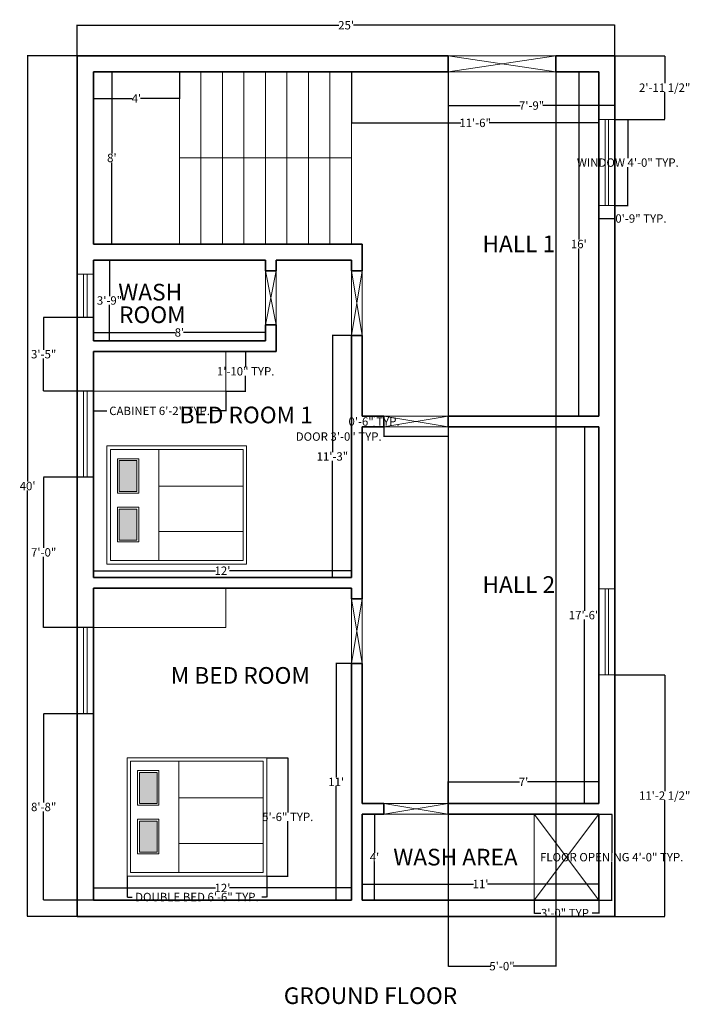
# Model space of a CAD drawing. Units: inches. Extents: x 292 to 2219, y -44 to 516.
# Tile 2 of 4: x 526 to 900, y -44 to 505. Entities that reach past the tile are written whole.
import ezdxf

# ---------------------------------------------------------------- set-up
doc = ezdxf.new("R2010")
doc.units = ezdxf.units.IN
doc.header["$MEASUREMENT"] = 0
for name, color, linetype, lineweight in [('A-ANNO-DIMS', 2, 'Continuous', 13), ('A-ANNO-TEXT', 7, 'Continuous', 25), ('A-AREA-IDEN', 7, 'Continuous', 18), ('A-DOOR', 34, 'Continuous', 20), ('A-FLOR-CASE', 9, 'Continuous', 18), ('A-FLOR-OPEN', 7, 'Continuous', 18), ('A-FLOR-STRS', 7, 'Continuous', 18), ('A-FURN', 8, 'Continuous', 18), ('A-GLAZ', 34, 'Continuous', 18), ('A-WALL', 7, 'Continuous', 35)]:
    doc.layers.add(name, color=color, linetype=linetype, lineweight=lineweight)
doc.styles.get("Standard").update_dxf_attribs({"font": 'arial.ttf'})
doc.dimstyles.get("Standard").update_dxf_attribs({"dimtxt": 4.68, "dimasz": 0.18, "dimexe": 0.18, "dimexo": 0.0625, "dimgap": 0.09, "dimtad": 0, "dimtih": 1, "dimtoh": 1, "dimdec": 0, "dimzin": 0, "dimdsep": 46, "dimlunit": 3, "dimtxsty": 'Standard', "dimcen": 0.09, "dimadec": 0, "dimazin": 0, "dimtfac": 1, "dimtdec": 0, "dimtofl": 0, "dimtmove": 0, "dimatfit": 3, "dimfxl": 1, "dimtolj": 1, "dimtzin": 0, "dimarcsym": 0})

# ---------------------------------------------------------------- blocks, each defined once
blk = doc.blocks.new('*D1')
at = {"layer": 'A-ANNO-DIMS', "color": 0, "lineweight": -2, "transparency": 16777216}
for p, q in [((558.22, 484.82), (530.37, 484.82)), ((530.55, 484.64), (530.55, 247.3)), ((530.55, 5), (530.55, 242.34)), ((558.22, 4.82), (530.37, 4.82))]:
    blk.add_line(p, q, dxfattribs=at)
at = {"layer": 'A-ANNO-DIMS', "color": 0, "transparency": 16777216}
for points in [[(530.52, 484.64), (530.58, 484.64), (530.55, 484.82)], [(530.52, 5), (530.58, 5), (530.55, 4.82)]]:
    blk.add_solid(points, dxfattribs=at)
at = {"layer": 'Defpoints', "color": 0, "transparency": 16777216}
for p in [(530.55, 484.82), (558.28, 484.82), (558.28, 4.82)]:
    blk.add_point(p, dxfattribs=at)
at = {"layer": 'A-ANNO-DIMS', "color": 0, "transparency": 16777216, "insert": (530.55, 244.82), "char_height": 4.68, "attachment_point": 5}
blk.add_mtext("\\A1;40'", dxfattribs=at)
blk = doc.blocks.new('*D2')
at = {"layer": 'A-ANNO-DIMS', "color": 0, "lineweight": -2, "transparency": 16777216}
for p, q in [((558.28, 484.88), (558.28, 502.04)), ((558.46, 501.86), (704.18, 501.86)), ((858.1, 501.86), (712.38, 501.86)), ((858.28, 484.88), (858.28, 502.04))]:
    blk.add_line(p, q, dxfattribs=at)
at = {"layer": 'A-ANNO-DIMS', "color": 0, "transparency": 16777216}
for points in [[(558.46, 501.89), (558.46, 501.83), (558.28, 501.86)], [(858.1, 501.89), (858.1, 501.83), (858.28, 501.86)]]:
    blk.add_solid(points, dxfattribs=at)
at = {"layer": 'Defpoints', "color": 0, "transparency": 16777216}
for p in [(858.28, 501.86), (558.28, 484.82), (858.28, 484.82)]:
    blk.add_point(p, dxfattribs=at)
at = {"layer": 'A-ANNO-DIMS', "color": 0, "transparency": 16777216, "insert": (708.28, 501.86), "char_height": 4.68, "attachment_point": 5}
blk.add_mtext("\\A1;25'", dxfattribs=at)
blk = doc.blocks.new('*D3')
at = {"layer": 'A-ANNO-DIMS', "color": 0, "lineweight": -2, "transparency": 16777216}
for p, q in [((849.22, 475.82), (837.97, 475.82)), ((838.15, 475.64), (838.15, 382.3)), ((838.15, 284), (838.15, 377.34)), ((849.22, 283.82), (837.97, 283.82))]:
    blk.add_line(p, q, dxfattribs=at)
at = {"layer": 'A-ANNO-DIMS', "color": 0, "transparency": 16777216}
for points in [[(838.12, 475.64), (838.18, 475.64), (838.15, 475.82)], [(838.12, 284), (838.18, 284), (838.15, 283.82)]]:
    blk.add_solid(points, dxfattribs=at)
at = {"layer": 'Defpoints', "color": 0, "transparency": 16777216}
for p in [(849.28, 475.82), (838.15, 283.82), (849.28, 283.82)]:
    blk.add_point(p, dxfattribs=at)
at = {"layer": 'A-ANNO-DIMS', "color": 0, "transparency": 16777216, "insert": (838.15, 379.82), "char_height": 4.68, "attachment_point": 5}
blk.add_mtext("\\A1;16'", dxfattribs=at)
blk = doc.blocks.new('*D4')
at = {"layer": 'A-ANNO-DIMS', "color": 0, "lineweight": -2, "transparency": 16777216}
for p, q in [((711.28, 475.75), (711.28, 447.21)), ((849.28, 475.75), (849.28, 447.21)), ((711.46, 447.39), (772.37, 447.39)), ((849.1, 447.39), (788.19, 447.39))]:
    blk.add_line(p, q, dxfattribs=at)
at = {"layer": 'A-ANNO-DIMS', "color": 0, "transparency": 16777216}
for points in [[(711.46, 447.42), (711.46, 447.36), (711.28, 447.39)], [(849.1, 447.42), (849.1, 447.36), (849.28, 447.39)]]:
    blk.add_solid(points, dxfattribs=at)
at = {"layer": 'Defpoints', "color": 0, "transparency": 16777216}
for p in [(711.28, 475.82), (849.28, 475.82), (849.28, 447.39)]:
    blk.add_point(p, dxfattribs=at)
at = {"layer": 'A-ANNO-DIMS', "color": 0, "transparency": 16777216, "insert": (780.28, 447.39), "char_height": 4.68, "attachment_point": 5}
blk.add_mtext('\\A1;11\'-6"', dxfattribs=at)
blk = doc.blocks.new('*D5')
at = {"layer": 'A-ANNO-DIMS', "color": 0, "lineweight": -2, "transparency": 16777216}
for p, q in [((567.28, 475.75), (567.28, 460.8)), ((615.28, 475.75), (615.28, 460.8)), ((567.46, 460.98), (588.94, 460.98)), ((615.1, 460.98), (593.62, 460.98))]:
    blk.add_line(p, q, dxfattribs=at)
at = {"layer": 'A-ANNO-DIMS', "color": 0, "transparency": 16777216}
for points in [[(567.46, 461.01), (567.46, 460.95), (567.28, 460.98)], [(615.1, 461.01), (615.1, 460.95), (615.28, 460.98)]]:
    blk.add_solid(points, dxfattribs=at)
at = {"layer": 'Defpoints', "color": 0, "transparency": 16777216}
for p in [(567.28, 475.82), (615.28, 475.82), (615.28, 460.98)]:
    blk.add_point(p, dxfattribs=at)
at = {"layer": 'A-ANNO-DIMS', "color": 0, "transparency": 16777216, "insert": (591.28, 460.98), "char_height": 4.68, "attachment_point": 5}
blk.add_mtext("\\A1;4'", dxfattribs=at)
blk = doc.blocks.new('*D6')
at = {"layer": 'A-ANNO-DIMS', "color": 0, "lineweight": -2, "transparency": 16777216}
for p, q in [((567.34, 475.82), (577.74, 475.82)), ((577.56, 475.64), (577.56, 430.3)), ((577.56, 380), (577.56, 425.34)), ((567.34, 379.82), (577.74, 379.82))]:
    blk.add_line(p, q, dxfattribs=at)
at = {"layer": 'A-ANNO-DIMS', "color": 0, "transparency": 16777216}
for points in [[(577.53, 475.64), (577.59, 475.64), (577.56, 475.82)], [(577.53, 380), (577.59, 380), (577.56, 379.82)]]:
    blk.add_solid(points, dxfattribs=at)
at = {"layer": 'Defpoints', "color": 0, "transparency": 16777216}
for p in [(567.28, 475.82), (567.28, 379.82), (577.56, 379.82)]:
    blk.add_point(p, dxfattribs=at)
at = {"layer": 'A-ANNO-DIMS', "color": 0, "transparency": 16777216, "insert": (577.56, 427.82), "char_height": 4.68, "attachment_point": 5}
blk.add_mtext("\\A1;8'", dxfattribs=at)
blk = doc.blocks.new('*D7')
at = {"layer": 'A-ANNO-DIMS', "color": 0, "lineweight": -2, "transparency": 16777216}
for p, q in [((567.28, 325.88), (567.28, 330.66)), ((567.46, 330.48), (613.03, 330.48)), ((663.1, 330.48), (617.52, 330.48)), ((663.28, 325.88), (663.28, 330.66))]:
    blk.add_line(p, q, dxfattribs=at)
at = {"layer": 'A-ANNO-DIMS', "color": 0, "transparency": 16777216}
for points in [[(567.46, 330.51), (567.46, 330.45), (567.28, 330.48)], [(663.1, 330.51), (663.1, 330.45), (663.28, 330.48)]]:
    blk.add_solid(points, dxfattribs=at)
at = {"layer": 'Defpoints', "color": 0, "transparency": 16777216}
for p in [(663.28, 330.48), (567.28, 325.82), (663.28, 325.82)]:
    blk.add_point(p, dxfattribs=at)
at = {"layer": 'A-ANNO-DIMS', "color": 0, "transparency": 16777216, "insert": (615.28, 330.48), "char_height": 4.68, "attachment_point": 5}
blk.add_mtext("\\A1;8'", dxfattribs=at)
blk = doc.blocks.new('*D8')
at = {"layer": 'A-ANNO-DIMS', "color": 0, "lineweight": -2, "transparency": 16777216}
for p, q in [((567.34, 370.82), (576.43, 370.82)), ((576.25, 370.64), (576.25, 350.8)), ((576.25, 326), (576.25, 345.84)), ((567.34, 325.82), (576.43, 325.82))]:
    blk.add_line(p, q, dxfattribs=at)
at = {"layer": 'A-ANNO-DIMS', "color": 0, "transparency": 16777216}
for points in [[(576.22, 370.64), (576.28, 370.64), (576.25, 370.82)], [(576.22, 326), (576.28, 326), (576.25, 325.82)]]:
    blk.add_solid(points, dxfattribs=at)
at = {"layer": 'Defpoints', "color": 0, "transparency": 16777216}
for p in [(567.28, 370.82), (576.25, 370.82), (567.28, 325.82)]:
    blk.add_point(p, dxfattribs=at)
at = {"layer": 'A-ANNO-DIMS', "color": 0, "transparency": 16777216, "insert": (576.25, 348.32), "char_height": 4.68, "attachment_point": 5}
blk.add_mtext('\\A1;3\'-9"', dxfattribs=at)
blk = doc.blocks.new('*D9')
at = {"layer": 'A-ANNO-DIMS', "color": 0, "lineweight": -2, "transparency": 16777216}
for p, q in [((711.22, 328.82), (700.45, 328.82)), ((700.63, 328.64), (700.63, 263.8)), ((700.63, 194), (700.63, 258.84)), ((711.22, 193.82), (700.45, 193.82))]:
    blk.add_line(p, q, dxfattribs=at)
at = {"layer": 'A-ANNO-DIMS', "color": 0, "transparency": 16777216}
for points in [[(700.6, 328.64), (700.66, 328.64), (700.63, 328.82)], [(700.6, 194), (700.66, 194), (700.63, 193.82)]]:
    blk.add_solid(points, dxfattribs=at)
at = {"layer": 'Defpoints', "color": 0, "transparency": 16777216}
for p in [(700.63, 328.82), (711.28, 328.82), (711.28, 193.82)]:
    blk.add_point(p, dxfattribs=at)
at = {"layer": 'A-ANNO-DIMS', "color": 0, "transparency": 16777216, "insert": (700.63, 261.32), "char_height": 4.68, "attachment_point": 5}
blk.add_mtext('\\A1;11\'-3"', dxfattribs=at)
blk = doc.blocks.new('*D10')
at = {"layer": 'A-ANNO-DIMS', "color": 0, "lineweight": -2, "transparency": 16777216}
for p, q in [((567.28, 193.88), (567.28, 197.79)), ((711.28, 193.88), (711.28, 197.79)), ((567.46, 197.61), (635.44, 197.61)), ((711.1, 197.61), (643.12, 197.61))]:
    blk.add_line(p, q, dxfattribs=at)
at = {"layer": 'A-ANNO-DIMS', "color": 0, "transparency": 16777216}
for points in [[(567.46, 197.64), (567.46, 197.58), (567.28, 197.61)], [(711.1, 197.64), (711.1, 197.58), (711.28, 197.61)]]:
    blk.add_solid(points, dxfattribs=at)
at = {"layer": 'Defpoints', "color": 0, "transparency": 16777216}
for p in [(567.28, 193.82), (711.28, 197.61), (711.28, 193.82)]:
    blk.add_point(p, dxfattribs=at)
at = {"layer": 'A-ANNO-DIMS', "color": 0, "transparency": 16777216, "insert": (639.28, 197.61), "char_height": 4.68, "attachment_point": 5}
blk.add_mtext("\\A1;12'", dxfattribs=at)
blk = doc.blocks.new('*D11')
at = {"layer": 'A-ANNO-DIMS', "color": 0, "lineweight": -2, "transparency": 16777216}
for p, q in [((567.28, 13.88), (567.28, 20.83)), ((567.46, 20.65), (635.44, 20.65)), ((711.1, 20.65), (643.12, 20.65)), ((711.28, 13.88), (711.28, 20.83))]:
    blk.add_line(p, q, dxfattribs=at)
at = {"layer": 'A-ANNO-DIMS', "color": 0, "transparency": 16777216}
for points in [[(567.46, 20.68), (567.46, 20.62), (567.28, 20.65)], [(711.1, 20.68), (711.1, 20.62), (711.28, 20.65)]]:
    blk.add_solid(points, dxfattribs=at)
at = {"layer": 'Defpoints', "color": 0, "transparency": 16777216}
for p in [(711.28, 20.65), (567.28, 13.82), (711.28, 13.82)]:
    blk.add_point(p, dxfattribs=at)
at = {"layer": 'A-ANNO-DIMS', "color": 0, "transparency": 16777216, "insert": (639.28, 20.65), "char_height": 4.68, "attachment_point": 5}
blk.add_mtext("\\A1;12'", dxfattribs=at)
blk = doc.blocks.new('*D12')
at = {"layer": 'A-ANNO-DIMS', "color": 0, "lineweight": -2, "transparency": 16777216}
for p, q in [((711.22, 145.82), (702.56, 145.82)), ((702.74, 145.64), (702.74, 82.26)), ((702.74, 14), (702.74, 77.38)), ((711.22, 13.82), (702.56, 13.82))]:
    blk.add_line(p, q, dxfattribs=at)
at = {"layer": 'A-ANNO-DIMS', "color": 0, "transparency": 16777216}
for points in [[(702.71, 145.64), (702.77, 145.64), (702.74, 145.82)], [(702.71, 14), (702.77, 14), (702.74, 13.82)]]:
    blk.add_solid(points, dxfattribs=at)
at = {"layer": 'Defpoints', "color": 0, "transparency": 16777216}
for p in [(702.74, 145.82), (711.28, 145.82), (711.28, 13.82)]:
    blk.add_point(p, dxfattribs=at)
at = {"layer": 'A-ANNO-DIMS', "color": 0, "transparency": 16777216, "insert": (702.74, 79.82), "char_height": 4.68, "attachment_point": 5}
blk.add_mtext("\\A1;11'", dxfattribs=at)
blk = doc.blocks.new('*D13')
at = {"layer": 'A-ANNO-DIMS', "color": 0, "lineweight": -2, "transparency": 16777216}
for p, q in [((717.28, 13.88), (717.28, 23.02)), ((717.46, 22.84), (779.44, 22.84)), ((849.1, 22.84), (787.12, 22.84)), ((849.28, 13.88), (849.28, 23.02))]:
    blk.add_line(p, q, dxfattribs=at)
at = {"layer": 'A-ANNO-DIMS', "color": 0, "transparency": 16777216}
for points in [[(717.46, 22.87), (717.46, 22.81), (717.28, 22.84)], [(849.1, 22.87), (849.1, 22.81), (849.28, 22.84)]]:
    blk.add_solid(points, dxfattribs=at)
at = {"layer": 'Defpoints', "color": 0, "transparency": 16777216}
for p in [(849.28, 22.84), (717.28, 13.82), (849.28, 13.82)]:
    blk.add_point(p, dxfattribs=at)
at = {"layer": 'A-ANNO-DIMS', "color": 0, "transparency": 16777216, "insert": (783.28, 22.84), "char_height": 4.68, "attachment_point": 5}
blk.add_mtext("\\A1;11'", dxfattribs=at)
blk = doc.blocks.new('*D14')
at = {"layer": 'A-ANNO-DIMS', "color": 0, "lineweight": -2, "transparency": 16777216}
for p, q in [((717.34, 61.82), (724.29, 61.82)), ((724.11, 61.64), (724.11, 40.25)), ((724.11, 14), (724.11, 35.39)), ((717.34, 13.82), (724.29, 13.82))]:
    blk.add_line(p, q, dxfattribs=at)
at = {"layer": 'A-ANNO-DIMS', "color": 0, "transparency": 16777216}
for points in [[(724.08, 61.64), (724.14, 61.64), (724.11, 61.82)], [(724.08, 14), (724.14, 14), (724.11, 13.82)]]:
    blk.add_solid(points, dxfattribs=at)
at = {"layer": 'Defpoints', "color": 0, "transparency": 16777216}
for p in [(717.28, 61.82), (717.28, 13.82), (724.11, 13.82)]:
    blk.add_point(p, dxfattribs=at)
at = {"layer": 'A-ANNO-DIMS', "color": 0, "transparency": 16777216, "insert": (724.11, 37.82), "char_height": 4.68, "attachment_point": 5}
blk.add_mtext("\\A1;4'", dxfattribs=at)
blk = doc.blocks.new('*D15')
at = {"layer": 'A-ANNO-DIMS', "color": 0, "lineweight": -2, "transparency": 16777216}
for p, q in [((849.22, 277.82), (841.19, 277.82)), ((841.37, 277.64), (841.37, 175.3)), ((841.37, 68), (841.37, 170.34)), ((849.22, 67.82), (841.19, 67.82))]:
    blk.add_line(p, q, dxfattribs=at)
at = {"layer": 'A-ANNO-DIMS', "color": 0, "transparency": 16777216}
for points in [[(841.34, 277.64), (841.4, 277.64), (841.37, 277.82)], [(841.34, 68), (841.4, 68), (841.37, 67.82)]]:
    blk.add_solid(points, dxfattribs=at)
at = {"layer": 'Defpoints', "color": 0, "transparency": 16777216}
for p in [(849.28, 277.82), (841.37, 67.82), (849.28, 67.82)]:
    blk.add_point(p, dxfattribs=at)
at = {"layer": 'A-ANNO-DIMS', "color": 0, "transparency": 16777216, "insert": (841.37, 172.82), "char_height": 4.68, "attachment_point": 5}
blk.add_mtext('\\A1;17\'-6"', dxfattribs=at)
blk = doc.blocks.new('*D16')
at = {"layer": 'A-ANNO-DIMS', "color": 0, "lineweight": -2, "transparency": 16777216}
for p, q in [((765.28, 67.88), (765.28, 79.96)), ((765.46, 79.78), (805.05, 79.78)), ((849.1, 79.78), (809.5, 79.78)), ((849.28, 67.88), (849.28, 79.96))]:
    blk.add_line(p, q, dxfattribs=at)
at = {"layer": 'A-ANNO-DIMS', "color": 0, "transparency": 16777216}
for points in [[(765.46, 79.81), (765.46, 79.75), (765.28, 79.78)], [(849.1, 79.81), (849.1, 79.75), (849.28, 79.78)]]:
    blk.add_solid(points, dxfattribs=at)
at = {"layer": 'Defpoints', "color": 0, "transparency": 16777216}
for p in [(849.28, 79.78), (765.28, 67.82), (849.28, 67.82)]:
    blk.add_point(p, dxfattribs=at)
at = {"layer": 'A-ANNO-DIMS', "color": 0, "transparency": 16777216, "insert": (807.28, 79.78), "char_height": 4.68, "attachment_point": 5}
blk.add_mtext("\\A1;7'", dxfattribs=at)
blk = doc.blocks.new('BED-DOUBLE')
h = blk.add_hatch(color=256)
h.dxf.hatch_style = 1
h.paths.add_polyline_path([(6.9, 40.51), (16.75, 40.51), (16.75, 57.79), (6.9, 57.79)])
h.paths.add_polyline_path([(16.75, 30.67), (6.9, 30.67), (6.9, 13.4), (16.75, 13.4)])
for p, q in [((0, 0), (0, 66)), ((0, 66), (78, 66)), ((78, 66), (78, 0)), ((2, 64), (76, 64)), ((2, 2), (2, 64)), ((29, 2), (29, 64)), ((76, 64), (76, 2)), ((76, 43.53), (29, 43.53)), ((76, 18.22), (29, 18.22)), ((78, 0), (0, 0)), ((76, 2), (2, 2))]:
    blk.add_line(p, q)
for points in [[(5.9, 58.79), (17.75, 58.79), (17.75, 39.51), (5.9, 39.51)], [(6.9, 57.79), (16.75, 57.79), (16.75, 40.51), (6.9, 40.51)], [(5.9, 31.67), (17.75, 31.67), (17.75, 12.4), (5.9, 12.4)], [(6.9, 30.67), (16.75, 30.67), (16.75, 13.4), (6.9, 13.4)]]:
    blk.add_lwpolyline(points, close=True)
blk = doc.blocks.new('WIN-48')
for p, q in [((0, 48), (9, 48)), ((0, 0), (0, 48)), ((3.5, 48), (3.5, 0)), ((5.5, 48), (5.5, 0)), ((9, 48), (9, 0)), ((9, 0), (0, 0))]:
    blk.add_line(p, q)
blk = doc.blocks.new('DOOR-36')
for p, q in [((0, 36), (6, 36)), ((0, 0), (6, 36)), ((6, 0), (0, 36)), ((0, 36), (0, 0)), ((6, 36), (6, 0)), ((0, 0), (6, 0))]:
    blk.add_line(p, q)
blk = doc.blocks.new('WIN-24')
for p, q in [((0, 24), (9, 24)), ((0, 24), (0, 0)), ((3.5, 24), (3.5, 0)), ((5.5, 24), (5.5, 0)), ((9, 24), (9, 0)), ((0, 0), (9, 0))]:
    blk.add_line(p, q)
blk = doc.blocks.new('DOOR-30')
for p, q in [((0, 30), (6, 30)), ((0, 30), (6, 0)), ((6, 30), (0, 0)), ((0, 0), (0, 30)), ((6, 0), (6, 30)), ((0, 0), (6, 0))]:
    blk.add_line(p, q)
blk = doc.blocks.new('FLOOR-OPENING-36X48')
for p, q in [((0, 48), (0, 0)), ((0, 48), (36, 0)), ((36, 48), (0, 0))]:
    blk.add_line(p, q)
blk = doc.blocks.new('BEDROOM-CABINET')
blk.add_lwpolyline([(0, 21.98), (73.86, 21.98), (73.86, 0), (0, 0)], close=True)
blk = doc.blocks.new('*D44')
at = {"layer": 'A-ANNO-DIMS', "color": 0, "lineweight": -2, "transparency": 16777216}
for p, q in [((858.34, 449.23), (865.66, 449.23)), ((865.48, 449.05), (865.48, 427.74)), ((865.48, 401.41), (865.48, 422.72)), ((858.34, 401.23), (865.66, 401.23))]:
    blk.add_line(p, q, dxfattribs=at)
at = {"layer": 'A-ANNO-DIMS', "color": 0, "transparency": 16777216}
for points in [[(865.45, 449.05), (865.51, 449.05), (865.48, 449.23)], [(865.45, 401.41), (865.51, 401.41), (865.48, 401.23)]]:
    blk.add_solid(points, dxfattribs=at)
at = {"layer": 'Defpoints', "color": 0, "transparency": 16777216}
for p in [(858.28, 449.23), (865.48, 449.23), (858.28, 401.23)]:
    blk.add_point(p, dxfattribs=at)
at = {"layer": 'A-ANNO-DIMS', "color": 0, "transparency": 16777216, "insert": (865.48, 425.23), "char_height": 4.68, "attachment_point": 5}
blk.add_mtext('\\A1;WINDOW 4\'-0" TYP.', dxfattribs=at)
blk = doc.blocks.new('*D45')
at = {"layer": 'A-ANNO-DIMS', "color": 0, "lineweight": -2, "transparency": 16777216}
for p, q in [((849.28, 401.17), (849.28, 393.85)), ((858.28, 401.17), (858.28, 393.85)), ((849.46, 394.03), (858.1, 394.03)), ((858.28, 394.03), (858.46, 394.03))]:
    blk.add_line(p, q, dxfattribs=at)
at = {"layer": 'A-ANNO-DIMS', "color": 0, "transparency": 16777216}
for points in [[(849.46, 394.06), (849.46, 394), (849.28, 394.03)], [(858.1, 394.06), (858.1, 394), (858.28, 394.03)]]:
    blk.add_solid(points, dxfattribs=at)
at = {"layer": 'Defpoints', "color": 0, "transparency": 16777216}
for p in [(849.28, 401.23), (858.28, 401.23), (858.28, 394.03)]:
    blk.add_point(p, dxfattribs=at)
at = {"layer": 'A-ANNO-DIMS', "color": 0, "transparency": 16777216, "insert": (872.81, 394.03), "char_height": 4.68, "attachment_point": 5}
blk.add_mtext('\\A1;0\'-9" TYP.', dxfattribs=at)
blk = doc.blocks.new('*D48')
at = {"layer": 'A-ANNO-DIMS', "color": 0, "lineweight": -2, "transparency": 16777216}
for p, q in [((729.28, 277.75), (729.28, 272.24)), ((765.28, 277.75), (765.28, 272.24)), ((729.28, 272.42), (729.1, 272.42)), ((765.1, 272.42), (729.46, 272.42))]:
    blk.add_line(p, q, dxfattribs=at)
at = {"layer": 'A-ANNO-DIMS', "color": 0, "transparency": 16777216}
for points in [[(729.46, 272.45), (729.46, 272.39), (729.28, 272.42)], [(765.1, 272.45), (765.1, 272.39), (765.28, 272.42)]]:
    blk.add_solid(points, dxfattribs=at)
at = {"layer": 'Defpoints', "color": 0, "transparency": 16777216}
for p in [(729.28, 277.82), (765.28, 277.82), (729.28, 272.42)]:
    blk.add_point(p, dxfattribs=at)
at = {"layer": 'A-ANNO-DIMS', "color": 0, "transparency": 16777216, "insert": (704.15, 272.42), "char_height": 4.68, "attachment_point": 5}
blk.add_mtext('\\A1;DOOR 3\'-0" TYP.', dxfattribs=at)
blk = doc.blocks.new('*D49')
at = {"layer": 'A-ANNO-DIMS', "color": 0, "lineweight": -2, "transparency": 16777216}
for p, q in [((729.22, 283.82), (723.7, 283.82)), ((723.88, 283.64), (723.88, 283.3)), ((729.22, 277.82), (723.7, 277.82)), ((723.88, 278), (723.88, 278.34))]:
    blk.add_line(p, q, dxfattribs=at)
at = {"layer": 'A-ANNO-DIMS', "color": 0, "transparency": 16777216}
for points in [[(723.85, 283.64), (723.91, 283.64), (723.88, 283.82)], [(723.85, 278), (723.91, 278), (723.88, 277.82)]]:
    blk.add_solid(points, dxfattribs=at)
at = {"layer": 'Defpoints', "color": 0, "transparency": 16777216}
for p in [(723.88, 283.82), (729.28, 283.82), (729.28, 277.82)]:
    blk.add_point(p, dxfattribs=at)
at = {"layer": 'A-ANNO-DIMS', "color": 0, "transparency": 16777216, "insert": (723.88, 280.82), "char_height": 4.68, "attachment_point": 5}
blk.add_mtext('\\A1;0\'-6" TYP.', dxfattribs=at)
blk = doc.blocks.new('*D52')
at = {"layer": 'A-ANNO-DIMS', "color": 0, "lineweight": -2, "transparency": 16777216}
for p, q in [((586.02, 27.24), (586.02, 15.42)), ((664.02, 27.24), (664.02, 15.42)), ((586.2, 15.6), (588.8, 15.6)), ((663.84, 15.6), (661.24, 15.6))]:
    blk.add_line(p, q, dxfattribs=at)
at = {"layer": 'A-ANNO-DIMS', "color": 0, "transparency": 16777216}
for points in [[(586.2, 15.63), (586.2, 15.57), (586.02, 15.6)], [(663.84, 15.63), (663.84, 15.57), (664.02, 15.6)]]:
    blk.add_solid(points, dxfattribs=at)
at = {"layer": 'Defpoints', "color": 0, "transparency": 16777216}
for p in [(586.02, 27.3), (664.02, 27.3), (664.02, 15.6)]:
    blk.add_point(p, dxfattribs=at)
at = {"layer": 'A-ANNO-DIMS', "color": 0, "transparency": 16777216, "insert": (625.02, 15.6), "char_height": 4.68, "attachment_point": 5}
blk.add_mtext('\\A1;DOUBLE BED 6\'-6" TYP.', dxfattribs=at)
blk = doc.blocks.new('*D53')
at = {"layer": 'A-ANNO-DIMS', "color": 0, "lineweight": -2, "transparency": 16777216}
for p, q in [((664.08, 93.3), (675.9, 93.3)), ((675.72, 93.12), (675.72, 62.78)), ((675.72, 27.48), (675.72, 57.82)), ((664.08, 27.3), (675.9, 27.3))]:
    blk.add_line(p, q, dxfattribs=at)
at = {"layer": 'A-ANNO-DIMS', "color": 0, "transparency": 16777216}
for points in [[(675.69, 93.12), (675.75, 93.12), (675.72, 93.3)], [(675.69, 27.48), (675.75, 27.48), (675.72, 27.3)]]:
    blk.add_solid(points, dxfattribs=at)
at = {"layer": 'Defpoints', "color": 0, "transparency": 16777216}
for p in [(664.02, 93.3), (675.72, 93.3), (664.02, 27.3)]:
    blk.add_point(p, dxfattribs=at)
at = {"layer": 'A-ANNO-DIMS', "color": 0, "transparency": 16777216, "insert": (675.72, 60.3), "char_height": 4.68, "attachment_point": 5}
blk.add_mtext('\\A1;5\'-6" TYP.', dxfattribs=at)
blk = doc.blocks.new('*D54')
at = {"layer": 'A-ANNO-DIMS', "color": 0, "lineweight": -2, "transparency": 16777216}
for p, q in [((567.28, 297.77), (567.28, 286.57)), ((641.14, 297.77), (641.14, 286.57)), ((567.46, 286.75), (574.81, 286.75)), ((640.96, 286.75), (633.61, 286.75))]:
    blk.add_line(p, q, dxfattribs=at)
at = {"layer": 'A-ANNO-DIMS', "color": 0, "transparency": 16777216}
for points in [[(567.46, 286.78), (567.46, 286.72), (567.28, 286.75)], [(640.96, 286.78), (640.96, 286.72), (641.14, 286.75)]]:
    blk.add_solid(points, dxfattribs=at)
at = {"layer": 'Defpoints', "color": 0, "transparency": 16777216}
for p in [(567.28, 297.83), (641.14, 297.83), (641.14, 286.75)]:
    blk.add_point(p, dxfattribs=at)
at = {"layer": 'A-ANNO-DIMS', "color": 0, "transparency": 16777216, "insert": (604.21, 286.75), "char_height": 4.68, "attachment_point": 5}
blk.add_mtext('\\A1;CABINET 6\'-2" TYP.', dxfattribs=at)
blk = doc.blocks.new('*D55')
at = {"layer": 'A-ANNO-DIMS', "color": 0, "lineweight": -2, "transparency": 16777216}
for p, q in [((641.2, 319.82), (652.4, 319.82)), ((652.22, 319.64), (652.22, 311.3)), ((652.22, 298.01), (652.22, 306.34)), ((641.2, 297.83), (652.4, 297.83))]:
    blk.add_line(p, q, dxfattribs=at)
at = {"layer": 'A-ANNO-DIMS', "color": 0, "transparency": 16777216}
for points in [[(652.19, 319.64), (652.25, 319.64), (652.22, 319.82)], [(652.19, 298.01), (652.25, 298.01), (652.22, 297.83)]]:
    blk.add_solid(points, dxfattribs=at)
at = {"layer": 'Defpoints', "color": 0, "transparency": 16777216}
for p in [(641.14, 319.82), (652.22, 319.82), (641.14, 297.83)]:
    blk.add_point(p, dxfattribs=at)
at = {"layer": 'A-ANNO-DIMS', "color": 0, "transparency": 16777216, "insert": (652.22, 308.82), "char_height": 4.68, "attachment_point": 5}
blk.add_mtext('\\A1;1\'-10" TYP.', dxfattribs=at)
blk = doc.blocks.new('*D56')
at = {"layer": 'A-ANNO-DIMS', "color": 0, "lineweight": -2, "transparency": 16777216}
for p, q in [((849.34, 61.82), (856.66, 61.82)), ((856.48, 61.64), (856.48, 40.33)), ((856.48, 14), (856.48, 35.3)), ((849.34, 13.82), (856.66, 13.82))]:
    blk.add_line(p, q, dxfattribs=at)
at = {"layer": 'A-ANNO-DIMS', "color": 0, "transparency": 16777216}
for points in [[(856.45, 61.64), (856.51, 61.64), (856.48, 61.82)], [(856.45, 14), (856.51, 14), (856.48, 13.82)]]:
    blk.add_solid(points, dxfattribs=at)
at = {"layer": 'Defpoints', "color": 0, "transparency": 16777216}
for p in [(849.28, 61.82), (856.48, 61.82), (849.28, 13.82)]:
    blk.add_point(p, dxfattribs=at)
at = {"layer": 'A-ANNO-DIMS', "color": 0, "transparency": 16777216, "insert": (856.48, 37.82), "char_height": 4.68, "attachment_point": 5}
blk.add_mtext('\\A1;FLOOR OPENING 4\'-0" TYP.', dxfattribs=at)
blk = doc.blocks.new('*D57')
at = {"layer": 'A-ANNO-DIMS', "color": 0, "lineweight": -2, "transparency": 16777216}
for p, q in [((813.28, 13.75), (813.28, 6.44)), ((849.28, 13.75), (849.28, 6.44)), ((813.46, 6.62), (816.93, 6.62)), ((849.1, 6.62), (845.63, 6.62))]:
    blk.add_line(p, q, dxfattribs=at)
at = {"layer": 'A-ANNO-DIMS', "color": 0, "transparency": 16777216}
for points in [[(813.46, 6.65), (813.46, 6.59), (813.28, 6.62)], [(849.1, 6.65), (849.1, 6.59), (849.28, 6.62)]]:
    blk.add_solid(points, dxfattribs=at)
at = {"layer": 'Defpoints', "color": 0, "transparency": 16777216}
for p in [(813.28, 13.82), (849.28, 13.82), (849.28, 6.62)]:
    blk.add_point(p, dxfattribs=at)
at = {"layer": 'A-ANNO-DIMS', "color": 0, "transparency": 16777216, "insert": (831.28, 6.62), "char_height": 4.68, "attachment_point": 5}
blk.add_mtext('\\A1;3\'-0" TYP.', dxfattribs=at)
blk = doc.blocks.new('*D58')
at = {"layer": 'A-ANNO-DIMS', "color": 0, "lineweight": -2, "transparency": 16777216}
for p, q in [((765.28, 475.75), (765.28, -23.14)), ((825.28, 475.75), (825.28, -23.14)), ((765.46, -22.96), (788.97, -22.96)), ((825.1, -22.96), (801.59, -22.96))]:
    blk.add_line(p, q, dxfattribs=at)
at = {"layer": 'A-ANNO-DIMS', "color": 0, "transparency": 16777216}
for points in [[(765.46, -22.93), (765.46, -22.99), (765.28, -22.96)], [(825.1, -22.93), (825.1, -22.99), (825.28, -22.96)]]:
    blk.add_solid(points, dxfattribs=at)
at = {"layer": 'Defpoints', "color": 0, "transparency": 16777216}
for p in [(765.28, 475.82), (825.28, 475.82), (825.28, -22.96)]:
    blk.add_point(p, dxfattribs=at)
at = {"layer": 'A-ANNO-DIMS', "color": 0, "transparency": 16777216, "insert": (795.28, -22.96), "char_height": 4.68, "attachment_point": 5}
blk.add_mtext('\\A1;5\'-0"', dxfattribs=at)
blk = doc.blocks.new('*D59')
at = {"layer": 'A-ANNO-DIMS', "color": 0, "lineweight": -2, "transparency": 16777216}
for p, q in [((765.28, 484.75), (765.28, 456.86)), ((858.28, 484.75), (858.28, 456.86)), ((765.46, 457.04), (805.49, 457.04)), ((858.1, 457.04), (818.07, 457.04))]:
    blk.add_line(p, q, dxfattribs=at)
at = {"layer": 'A-ANNO-DIMS', "color": 0, "transparency": 16777216}
for points in [[(765.46, 457.07), (765.46, 457.01), (765.28, 457.04)], [(858.1, 457.07), (858.1, 457.01), (858.28, 457.04)]]:
    blk.add_solid(points, dxfattribs=at)
at = {"layer": 'Defpoints', "color": 0, "transparency": 16777216}
for p in [(765.28, 484.82), (858.28, 484.82), (765.28, 457.04)]:
    blk.add_point(p, dxfattribs=at)
at = {"layer": 'A-ANNO-DIMS', "color": 0, "transparency": 16777216, "insert": (811.78, 457.04), "char_height": 4.68, "attachment_point": 5}
blk.add_mtext('\\A1;7\'-9"', dxfattribs=at)
blk = doc.blocks.new('*D60')
at = {"layer": 'A-ANNO-DIMS', "color": 0, "lineweight": -2, "transparency": 16777216}
for p, q in [((567.22, 117.83), (539.32, 117.83)), ((539.5, 117.65), (539.5, 68.3)), ((539.5, 14), (539.5, 63.34)), ((567.22, 13.82), (539.32, 13.82))]:
    blk.add_line(p, q, dxfattribs=at)
at = {"layer": 'A-ANNO-DIMS', "color": 0, "transparency": 16777216}
for points in [[(539.47, 117.65), (539.53, 117.65), (539.5, 117.83)], [(539.47, 14), (539.53, 14), (539.5, 13.82)]]:
    blk.add_solid(points, dxfattribs=at)
at = {"layer": 'Defpoints', "color": 0, "transparency": 16777216}
for p in [(539.5, 117.83), (567.28, 117.83), (567.28, 13.82)]:
    blk.add_point(p, dxfattribs=at)
at = {"layer": 'A-ANNO-DIMS', "color": 0, "transparency": 16777216, "insert": (539.5, 65.82), "char_height": 4.68, "attachment_point": 5}
blk.add_mtext('\\A1;8\'-8"', dxfattribs=at)
blk = doc.blocks.new('*D61')
at = {"layer": 'A-ANNO-DIMS', "color": 0, "lineweight": -2, "transparency": 16777216}
for p, q in [((567.22, 249.83), (539.32, 249.83)), ((539.5, 249.65), (539.5, 210.31)), ((539.5, 166.01), (539.5, 205.35)), ((567.22, 165.83), (539.32, 165.83))]:
    blk.add_line(p, q, dxfattribs=at)
at = {"layer": 'A-ANNO-DIMS', "color": 0, "transparency": 16777216}
for points in [[(539.47, 249.65), (539.53, 249.65), (539.5, 249.83)], [(539.47, 166.01), (539.53, 166.01), (539.5, 165.83)]]:
    blk.add_solid(points, dxfattribs=at)
at = {"layer": 'Defpoints', "color": 0, "transparency": 16777216}
for p in [(539.5, 249.83), (567.28, 249.83), (567.28, 165.83)]:
    blk.add_point(p, dxfattribs=at)
at = {"layer": 'A-ANNO-DIMS', "color": 0, "transparency": 16777216, "insert": (539.5, 207.83), "char_height": 4.68, "attachment_point": 5}
blk.add_mtext('\\A1;7\'-0"', dxfattribs=at)
blk = doc.blocks.new('*D62')
at = {"layer": 'A-ANNO-DIMS', "color": 0, "lineweight": -2, "transparency": 16777216}
for p, q in [((567.22, 338.92), (539.32, 338.92)), ((539.5, 338.74), (539.5, 320.86)), ((539.5, 298.01), (539.5, 315.89)), ((567.22, 297.83), (539.32, 297.83))]:
    blk.add_line(p, q, dxfattribs=at)
at = {"layer": 'A-ANNO-DIMS', "color": 0, "transparency": 16777216}
for points in [[(539.47, 338.74), (539.53, 338.74), (539.5, 338.92)], [(539.47, 298.01), (539.53, 298.01), (539.5, 297.83)]]:
    blk.add_solid(points, dxfattribs=at)
at = {"layer": 'Defpoints', "color": 0, "transparency": 16777216}
for p in [(539.5, 338.92), (567.28, 338.92), (567.28, 297.83)]:
    blk.add_point(p, dxfattribs=at)
at = {"layer": 'A-ANNO-DIMS', "color": 0, "transparency": 16777216, "insert": (539.5, 318.37), "char_height": 4.68, "attachment_point": 5}
blk.add_mtext('\\A1;3\'-5"', dxfattribs=at)
blk = doc.blocks.new('*D63')
at = {"layer": 'A-ANNO-DIMS', "color": 0, "lineweight": -2, "transparency": 16777216}
for p, q in [((858.34, 139.48), (886.23, 139.48)), ((886.05, 139.3), (886.05, 74.66)), ((886.05, 5), (886.05, 69.64)), ((858.34, 4.82), (886.23, 4.82))]:
    blk.add_line(p, q, dxfattribs=at)
at = {"layer": 'A-ANNO-DIMS', "color": 0, "transparency": 16777216}
for points in [[(886.02, 139.3), (886.08, 139.3), (886.05, 139.48)], [(886.02, 5), (886.08, 5), (886.05, 4.82)]]:
    blk.add_solid(points, dxfattribs=at)
at = {"layer": 'Defpoints', "color": 0, "transparency": 16777216}
for p in [(858.28, 139.48), (886.05, 139.48), (858.28, 4.82)]:
    blk.add_point(p, dxfattribs=at)
at = {"layer": 'A-ANNO-DIMS', "color": 0, "transparency": 16777216, "insert": (886.05, 72.15), "char_height": 4.68, "attachment_point": 5}
blk.add_mtext('\\A1;11\'-2 1/2"', dxfattribs=at)
blk = doc.blocks.new('*D64')
at = {"layer": 'A-ANNO-DIMS', "color": 0, "lineweight": -2, "transparency": 16777216}
for p, q in [((858.34, 484.82), (886.23, 484.82)), ((886.05, 484.64), (886.05, 469.53)), ((886.05, 449.41), (886.05, 464.51)), ((858.34, 449.23), (886.23, 449.23))]:
    blk.add_line(p, q, dxfattribs=at)
at = {"layer": 'A-ANNO-DIMS', "color": 0, "transparency": 16777216}
for points in [[(886.02, 484.64), (886.08, 484.64), (886.05, 484.82)], [(886.02, 449.41), (886.08, 449.41), (886.05, 449.23)]]:
    blk.add_solid(points, dxfattribs=at)
at = {"layer": 'Defpoints', "color": 0, "transparency": 16777216}
for p in [(858.28, 484.82), (886.05, 484.82), (858.28, 449.23)]:
    blk.add_point(p, dxfattribs=at)
at = {"layer": 'A-ANNO-DIMS', "color": 0, "transparency": 16777216, "insert": (886.05, 467.02), "char_height": 4.68, "attachment_point": 5}
blk.add_mtext('\\A1;2\'-11 1/2"', dxfattribs=at)

msp = doc.modelspace()

# ---------------------------------------------------------------- linework, layer by layer
at = {"layer": 'A-DOOR'}
for p, q in [((765.28, 475.82), (765.28, 484.82)), ((765.28, 484.82), (825.28, 475.82)), ((765.28, 475.82), (825.28, 484.82)), ((825.28, 484.82), (765.28, 484.82)), ((825.28, 475.82), (825.28, 484.82)), ((825.28, 475.82), (765.28, 475.82))]:
    msp.add_line(p, q, dxfattribs=at)
at = {"layer": 'A-FLOR-STRS'}
for p, q in [((615.28, 379.82), (615.28, 475.82)), ((627.28, 379.82), (627.28, 475.82)), ((639.28, 379.82), (639.28, 475.82)), ((651.28, 379.82), (651.28, 475.82)), ((663.28, 379.82), (663.28, 475.82)), ((675.28, 379.82), (675.28, 475.82)), ((687.28, 379.82), (687.28, 475.82)), ((699.28, 379.82), (699.28, 475.82)), ((711.28, 379.82), (711.28, 475.82)), ((615.28, 427.82), (711.28, 427.82))]:
    msp.add_line(p, q, dxfattribs=at)
at = {"layer": 'A-WALL'}
for p, q in [((558.28, 4.82), (558.28, 484.82)), ((558.28, 484.82), (765.28, 484.82)), ((765.28, 475.82), (765.28, 484.82)), ((825.28, 475.82), (825.28, 484.82)), ((825.28, 484.82), (858.28, 484.82)), ((858.28, 484.82), (858.28, 4.82)), ((567.28, 475.82), (765.28, 475.82)), ((567.28, 379.82), (567.28, 475.82)), ((825.28, 475.82), (849.28, 475.82)), ((849.28, 475.82), (849.28, 283.82)), ((567.28, 379.82), (717.28, 379.82)), ((717.28, 364.82), (717.28, 379.82)), ((567.28, 370.82), (663.28, 370.82)), ((567.28, 325.82), (567.28, 370.82)), ((663.28, 364.82), (663.28, 370.82)), ((669.28, 370.82), (711.28, 370.82)), ((669.28, 364.82), (669.28, 370.82)), ((711.28, 364.82), (711.28, 370.82)), ((663.28, 364.82), (669.28, 364.82)), ((711.28, 364.82), (717.28, 364.82)), ((663.28, 325.82), (663.28, 334.82)), ((663.28, 334.82), (669.28, 334.82)), ((669.28, 319.82), (669.28, 334.82)), ((567.28, 325.82), (663.28, 325.82)), ((711.28, 193.82), (711.28, 328.82)), ((711.28, 328.82), (717.28, 328.82)), ((717.28, 283.82), (717.28, 328.82)), ((567.28, 319.82), (669.28, 319.82)), ((567.28, 193.82), (567.28, 319.82)), ((717.28, 283.82), (729.28, 283.82)), ((729.28, 283.82), (729.28, 277.82)), ((765.28, 283.82), (765.28, 277.82)), ((765.28, 283.82), (849.28, 283.82)), ((717.28, 277.82), (729.28, 277.82)), ((717.28, 181.82), (717.28, 277.82)), ((765.28, 277.82), (849.28, 277.82)), ((849.28, 277.82), (849.28, 67.82)), ((567.28, 193.82), (711.28, 193.82)), ((567.28, 13.82), (567.28, 187.82)), ((567.28, 187.82), (711.28, 187.82)), ((711.28, 181.82), (711.28, 187.82)), ((711.28, 181.82), (717.28, 181.82)), ((711.28, 13.82), (711.28, 145.82)), ((711.28, 145.82), (717.28, 145.82)), ((717.28, 67.82), (717.28, 145.82)), ((717.28, 67.82), (729.28, 67.82)), ((729.28, 67.82), (729.28, 61.82)), ((765.28, 67.82), (765.28, 61.82)), ((765.28, 67.82), (849.28, 67.82)), ((717.28, 13.82), (717.28, 61.82)), ((717.28, 61.82), (729.28, 61.82)), ((765.28, 61.82), (849.28, 61.82)), ((849.28, 61.82), (849.28, 13.82)), ((567.28, 13.82), (711.28, 13.82)), ((717.28, 13.82), (849.28, 13.82)), ((558.28, 4.82), (858.28, 4.82))]:
    msp.add_line(p, q, dxfattribs=at)

# ---------------------------------------------------------------- block references
at = {"layer": 'A-DOOR'}
for name, p in [('DOOR-30', (663.28, 334.82)), ('DOOR-36', (711.28, 328.82)), ('DOOR-36', (711.28, 145.82))]:
    msp.add_blockref(name, p, dxfattribs=at)
for p, rotation in [((765.28, 277.82), 90.00000000000048), ((765.28, 61.82), 90.00000000000067)]:
    msp.add_blockref('DOOR-36', p, dxfattribs=dict(at, rotation=rotation))
at = {"layer": 'A-FLOR-CASE'}
for p in [(567.28, 297.83), (567.28, 165.83)]:
    msp.add_blockref('BEDROOM-CABINET', p, dxfattribs=at)
at = {"layer": 'A-FLOR-OPEN'}
msp.add_blockref('FLOOR-OPENING-36X48', (813.28, 13.82), dxfattribs=at)
at = {"layer": 'A-FURN'}
for p in [(574.77, 201.29), (586.02, 27.3)]:
    msp.add_blockref('BED-DOUBLE', p, dxfattribs=at)
at = {"layer": 'A-GLAZ'}
for name, p in [('WIN-48', (849.28, 401.23)), ('WIN-24', (558.28, 338.92)), ('WIN-48', (558.28, 249.83)), ('WIN-48', (849.28, 139.48)), ('WIN-48', (558.28, 117.83))]:
    msp.add_blockref(name, p, dxfattribs=at)

# ---------------------------------------------------------------- texts
at = {"layer": 'A-ANNO-TEXT'}
msp.add_text('GROUND FLOOR', height=9.289, dxfattribs=at).set_placement((673.5, -44.08))
at = {"layer": 'A-AREA-IDEN'}
for s, p in [('HALL 1', (784.37, 375.26)), ('WASH ', (581.16, 348.32)), ('ROOM', (581.58, 335.74)), ('BED ROOM 1', (615.3, 279.82)), ('HALL 2', (784.37, 185.22)), ('M BED ROOM', (610.44, 134.55)), ('WASH AREA ', (734.63, 33.2))]:
    msp.add_text(s, height=9.289, dxfattribs=at).set_placement(p)

# ---------------------------------------------------------------- dimensions: what is measured, and where the dimension line sits
at = {"layer": 'A-ANNO-DIMS'}
for base, p1, p2, override, picture, middle in [((858.28, 501.86), (558.28, 484.82), (858.28, 484.82), {"dimclrd": 0, "dimclre": 0, "dimclrt": 0}, '*D2', (708.28, 501.86)), ((615.28, 460.98), (567.28, 475.82), (615.28, 475.82), {"dimclrd": 0, "dimclre": 0, "dimclrt": 0}, '*D5', (591.28, 460.98)), ((849.28, 447.39), (711.28, 475.82), (849.28, 475.82), {"dimclrd": 0, "dimclre": 0, "dimclrt": 0}, '*D4', (780.28, 447.39)), ((825.28, -22.96), (765.28, 475.82), (825.28, 475.82), {"dimdec": 1, "dimlfac": 1, "dimrnd": 0, "dimzin": 1, "dimdsep": 46, "dimlunit": 4, "dimfrac": 2}, '*D58', (795.28, -22.96)), ((663.28, 330.48), (567.28, 325.82), (663.28, 325.82), {"dimclrd": 0, "dimclre": 0, "dimclrt": 0}, '*D7', (615.28, 330.48)), ((711.28, 197.61), (567.28, 193.82), (711.28, 193.82), {"dimclrd": 0, "dimclre": 0, "dimclrt": 0}, '*D10', (639.28, 197.61)), ((849.28, 79.78), (765.28, 67.82), (849.28, 67.82), {"dimclrd": 0, "dimclre": 0, "dimclrt": 0}, '*D16', (807.28, 79.78)), ((711.28, 20.65), (567.28, 13.82), (711.28, 13.82), {"dimclrd": 0, "dimclre": 0, "dimclrt": 0}, '*D11', (639.28, 20.65)), ((849.28, 22.84), (717.28, 13.82), (849.28, 13.82), {"dimclrd": 0, "dimclre": 0, "dimclrt": 0}, '*D13', (783.28, 22.84))]:
    dim = msp.add_linear_dim(base=base, p1=p1, p2=p2, dimstyle='Standard', override=override, dxfattribs=at)
    dim.commit()
    dim.dimension.update_dxf_attribs({"geometry": picture, "text_midpoint": middle})
for base, p1, p2, angle, override, picture, middle in [((530.55, 484.82), (558.28, 4.82), (558.28, 484.82), 90, {"dimclrd": 0, "dimclre": 0, "dimclrt": 0}, '*D1', (530.55, 244.82)), ((765.28, 457.04), (858.28, 484.82), (765.28, 484.82), 180, {"dimdec": 1, "dimlfac": 1, "dimrnd": 0, "dimzin": 1, "dimdsep": 46, "dimlunit": 4, "dimfrac": 2}, '*D59', (811.78, 457.04)), ((886.05, 484.82), (858.28, 449.23), (858.28, 484.82), 90, {"dimdec": 1, "dimlfac": 1, "dimrnd": 0, "dimzin": 1, "dimdsep": 46, "dimlunit": 4, "dimfrac": 2}, '*D64', (886.05, 467.02)), ((577.56, 379.82), (567.28, 475.82), (567.28, 379.82), 90, {"dimclrd": 0, "dimclre": 0, "dimclrt": 0}, '*D6', (577.56, 427.82)), ((838.15, 283.82), (849.28, 475.82), (849.28, 283.82), 90, {"dimclrd": 0, "dimclre": 0, "dimclrt": 0}, '*D3', (838.15, 379.82)), ((576.25, 370.82), (567.28, 325.82), (567.28, 370.82), 90, {"dimclrd": 0, "dimclre": 0, "dimclrt": 0}, '*D8', (576.25, 348.32)), ((539.5, 338.92), (567.28, 297.83), (567.28, 338.92), 90, {"dimdec": 1, "dimlfac": 1, "dimrnd": 0, "dimzin": 1, "dimdsep": 46, "dimlunit": 4, "dimfrac": 2}, '*D62', (539.5, 318.37)), ((700.63, 328.82), (711.28, 193.82), (711.28, 328.82), 90, {"dimclrd": 0, "dimclre": 0, "dimclrt": 0}, '*D9', (700.63, 261.32)), ((841.37, 67.82), (849.28, 277.82), (849.28, 67.82), 90, {"dimclrd": 0, "dimclre": 0, "dimclrt": 0}, '*D15', (841.37, 172.82)), ((539.5, 249.83), (567.28, 165.83), (567.28, 249.83), 90, {"dimdec": 1, "dimlfac": 1, "dimrnd": 0, "dimzin": 1, "dimdsep": 46, "dimlunit": 4, "dimfrac": 2}, '*D61', (539.5, 207.83)), ((702.74, 145.82), (711.28, 13.82), (711.28, 145.82), 90, {"dimclrd": 0, "dimclre": 0, "dimclrt": 0}, '*D12', (702.74, 79.82)), ((886.05, 139.48), (858.28, 4.82), (858.28, 139.48), 90, {"dimdec": 1, "dimlfac": 1, "dimrnd": 0, "dimzin": 1, "dimdsep": 46, "dimlunit": 4, "dimfrac": 2}, '*D63', (886.05, 72.15)), ((539.5, 117.83), (567.28, 13.82), (567.28, 117.83), 90, {"dimdec": 1, "dimlfac": 1, "dimrnd": 0, "dimzin": 1, "dimdsep": 46, "dimlunit": 4, "dimfrac": 2}, '*D60', (539.5, 65.82)), ((724.11, 13.82), (717.28, 61.82), (717.28, 13.82), 90, {"dimclrd": 0, "dimclre": 0, "dimclrt": 0}, '*D14', (724.11, 37.82))]:
    dim = msp.add_linear_dim(base=base, p1=p1, p2=p2, angle=angle, dimstyle='Standard', override=override, dxfattribs=at)
    dim.commit()
    dim.dimension.update_dxf_attribs({"geometry": picture, "text_midpoint": middle})
for base, p1, p2, angle, text, picture, middle in [((865.48, 449.23), (858.28, 401.23), (858.28, 449.23), 90, 'WINDOW <> TYP.', '*D44', (865.48, 425.23)), ((652.22, 319.82), (641.14, 297.83), (641.14, 319.82), 90, '<> TYP.', '*D55', (652.22, 308.82)), ((723.88, 283.82), (729.28, 277.82), (729.28, 283.82), 90, '<> TYP.', '*D49', (723.88, 280.82)), ((729.28, 272.42), (765.28, 277.82), (729.28, 277.82), 180, 'DOOR <> TYP.', '*D48', (704.15, 272.42)), ((675.72, 93.3), (664.02, 27.3), (664.02, 93.3), 90, '<> TYP.', '*D53', (675.72, 60.3)), ((856.48, 61.82), (849.28, 13.82), (849.28, 61.82), 90, 'FLOOR OPENING <> TYP.', '*D56', (856.48, 37.82))]:
    dim = msp.add_linear_dim(base=base, p1=p1, p2=p2, angle=angle, text=text, dimstyle='Standard', override={"dimdec": 1, "dimlfac": 1, "dimrnd": 0, "dimzin": 1, "dimdsep": 46, "dimlunit": 4, "dimfrac": 2}, dxfattribs=at)
    dim.commit()
    dim.dimension.update_dxf_attribs({"geometry": picture, "text_midpoint": middle})
for base, p1, p2, text, picture, middle in [((858.28, 394.03), (849.28, 401.23), (858.28, 401.23), '<> TYP.', '*D45', (872.81, 394.03)), ((641.14, 286.75), (567.28, 297.83), (641.14, 297.83), 'CABINET <> TYP.', '*D54', (604.21, 286.75)), ((664.02, 15.6), (586.02, 27.3), (664.02, 27.3), 'DOUBLE BED <> TYP.', '*D52', (625.02, 15.6)), ((849.28, 6.62), (813.28, 13.82), (849.28, 13.82), '<> TYP.', '*D57', (831.28, 6.62))]:
    dim = msp.add_linear_dim(base=base, p1=p1, p2=p2, text=text, dimstyle='Standard', override={"dimdec": 1, "dimlfac": 1, "dimrnd": 0, "dimzin": 1, "dimdsep": 46, "dimlunit": 4, "dimfrac": 2}, dxfattribs=at)
    dim.commit()
    dim.dimension.update_dxf_attribs({"geometry": picture, "text_midpoint": middle})

doc.saveas('drawing.dxf')
